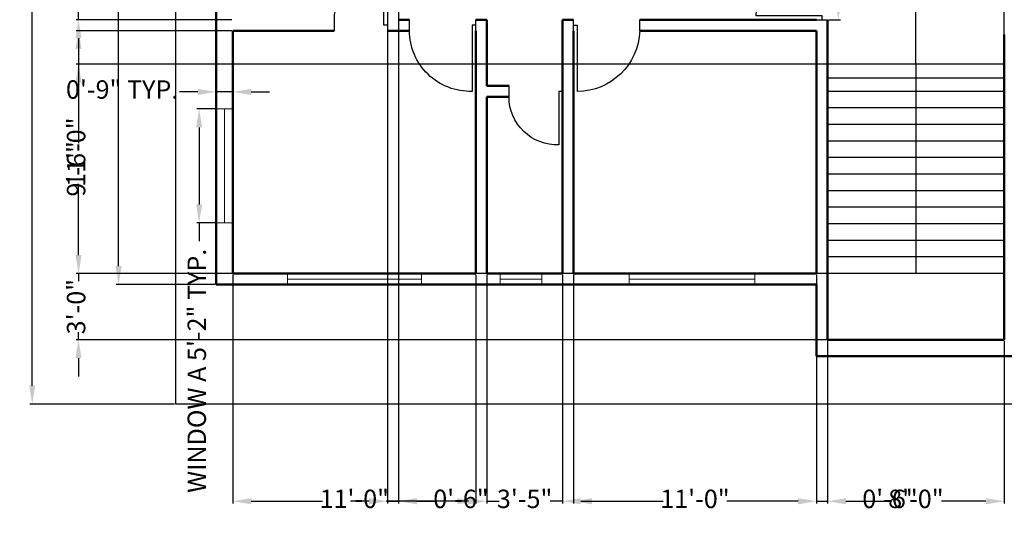
# Model space of a CAD drawing. Units: inches. Extents: x 3237 to 4201, y 2949 to 4053.
# Tile 1 of 5: x 3237 to 3772, y 2949 to 3217. Entities that reach past the tile are written whole.
import ezdxf

# ---------------------------------------------------------------- set-up
doc = ezdxf.new("R2010")
doc.units = ezdxf.units.IN
for name, color, linetype, lineweight in [('A-ANNO-DIMS', 2, 'Continuous', 18), ('A-DOOR', 3, 'Continuous', 25), ('A-FLOR-STRS', 7, 'Continuous', 25), ('A-GLAZ', 4, 'Continuous', 18), ('A-WALL', 7, 'Continuous', 50), ('C-PROP', 6, 'Continuous', 25)]:
    doc.layers.add(name, color=color, linetype=linetype, lineweight=lineweight)
doc.styles.get("Standard").update_dxf_attribs({"font": 'arial.ttf'})
doc.dimstyles.new('ISO-25', dxfattribs={"dimtxt": 10, "dimasz": 10, "dimexe": 1.25, "dimexo": 0.625, "dimtad": 0, "dimdec": 0, "dimlunit": 3, "dimtxsty": 'Standard', "dimcen": 2.5, "dimadec": 0, "dimazin": 0, "dimtfac": 1, "dimtdec": 0, "dimtmove": 0, "dimatfit": 3, "dimfxl": 1, "dimarcsym": 0})

# ---------------------------------------------------------------- blocks, each defined once
blk = doc.blocks.new('*D2')
at = {"layer": 'A-ANNO-DIMS', "color": 0, "lineweight": -2, "transparency": 16777216}
for p, q in [((3320.9, 3907.98), (3242.34, 3907.98)), ((3243.59, 3897.98), (3243.59, 3467.05)), ((3243.59, 3017.98), (3243.59, 3448.91)), ((3320.9, 3007.98), (3242.34, 3007.98))]:
    blk.add_line(p, q, dxfattribs=at)
at = {"layer": 'A-ANNO-DIMS', "color": 0, "transparency": 16777216}
for points in [[(3241.92, 3897.98), (3245.26, 3897.98), (3243.59, 3907.98)], [(3241.92, 3017.98), (3245.26, 3017.98), (3243.59, 3007.98)]]:
    blk.add_solid(points, dxfattribs=at)
at = {"layer": 'Defpoints', "color": 0, "transparency": 16777216}
for p in [(3321.52, 3907.98), (3243.59, 3007.98), (3321.52, 3007.98)]:
    blk.add_point(p, dxfattribs=at)
at = {"layer": 'A-ANNO-DIMS', "color": 0, "transparency": 16777216, "insert": (3243.59, 3457.98), "char_height": 10, "attachment_point": 5, "rotation": 90}
blk.add_mtext("75'", dxfattribs=at)
blk = doc.blocks.new('*D4')
at = {"layer": 'A-ANNO-DIMS', "color": 0, "lineweight": -2, "transparency": 16777216}
for p, q in [((3342.9, 3885.98), (3289.25, 3885.98)), ((3290.5, 3875.98), (3290.5, 3497.31)), ((3290.5, 3082.98), (3290.5, 3461.65)), ((3342.9, 3072.98), (3289.25, 3072.98))]:
    blk.add_line(p, q, dxfattribs=at)
at = {"layer": 'A-ANNO-DIMS', "color": 0, "transparency": 16777216}
for points in [[(3288.84, 3875.98), (3292.17, 3875.98), (3290.5, 3885.98)], [(3288.84, 3082.98), (3292.17, 3082.98), (3290.5, 3072.98)]]:
    blk.add_solid(points, dxfattribs=at)
at = {"layer": 'Defpoints', "color": 0, "transparency": 16777216}
for p in [(3343.52, 3885.98), (3290.5, 3072.98), (3343.52, 3072.98)]:
    blk.add_point(p, dxfattribs=at)
at = {"layer": 'A-ANNO-DIMS', "color": 0, "transparency": 16777216, "insert": (3290.5, 3479.48), "char_height": 10, "attachment_point": 5, "rotation": 90}
blk.add_mtext('67\'-9"', dxfattribs=at)
blk = doc.blocks.new('DOOR-36-OFFSET-A')
for p, q in [((2, 3), (2, 39)), ((0, 6), (0, 0)), ((36, 6), (36, 0)), ((0, 3), (2, 3))]:
    blk.add_line(p, q)
blk.add_arc((2, 4.98), 34.02, 1.7102, 90)
blk = doc.blocks.new('DOOR-29-OFFSET-B')
for p, q in [((27, 3), (27, 32)), ((0, 6), (0, 0)), ((29, 6), (29, 0)), ((29, 3), (27, 3))]:
    blk.add_line(p, q)
blk.add_arc((26.02, 6), 26.02, 87.8382, 180)
blk = doc.blocks.new('DOOR-36-OFFSET-B')
for p, q in [((34, 3), (34, 39)), ((0, 6), (0, 0)), ((36, 6), (36, 0)), ((36, 3), (34, 3))]:
    blk.add_line(p, q)
blk.add_arc((33.01, 6), 33.01, 88.2898, 180)
blk = doc.blocks.new('WIN-61p86IN')
for p, q in [((0, 61.86), (9, 61.86)), ((4.5, 0), (4.5, 61.86)), ((0, 0), (9, 0))]:
    blk.add_line(p, q)
blk = doc.blocks.new('*D22')
at = {"layer": 'A-ANNO-DIMS', "color": 0, "lineweight": -2, "transparency": 16777216}
for p, q in [((3681.37, 3252.98), (3681.37, 3262.98)), ((3676.15, 3252.98), (3682.62, 3252.98)), ((3681.37, 3226.98), (3681.37, 3242.98)), ((3676.15, 3216.98), (3682.62, 3216.98))]:
    blk.add_line(p, q, dxfattribs=at)
at = {"layer": 'A-ANNO-DIMS', "color": 0, "transparency": 16777216}
for points in [[(3679.71, 3242.98), (3683.04, 3242.98), (3681.37, 3252.98)], [(3679.71, 3226.98), (3683.04, 3226.98), (3681.37, 3216.98)]]:
    blk.add_solid(points, dxfattribs=at)
at = {"layer": 'Defpoints', "color": 0, "transparency": 16777216}
for p in [(3675.52, 3252.98), (3681.37, 3252.98), (3675.52, 3216.98)]:
    blk.add_point(p, dxfattribs=at)
at = {"layer": 'A-ANNO-DIMS', "color": 0, "transparency": 16777216, "insert": (3681.37, 3294.08), "char_height": 10, "attachment_point": 5, "rotation": 90}
blk.add_mtext('3\'-0" TYP.', dxfattribs=at)
blk = doc.blocks.new('*D27')
at = {"layer": 'A-ANNO-DIMS', "color": 0, "lineweight": -2, "transparency": 16777216}
for p, q in [((3342.9, 3168.43), (3332.99, 3168.43)), ((3334.24, 3158.43), (3334.24, 3116.57)), ((3342.9, 3106.57), (3332.99, 3106.57)), ((3334.24, 3106.57), (3334.24, 3096.57))]:
    blk.add_line(p, q, dxfattribs=at)
at = {"layer": 'A-ANNO-DIMS', "color": 0, "transparency": 16777216}
for points in [[(3332.58, 3158.43), (3335.91, 3158.43), (3334.24, 3168.43)], [(3332.58, 3116.57), (3335.91, 3116.57), (3334.24, 3106.57)]]:
    blk.add_solid(points, dxfattribs=at)
at = {"layer": 'Defpoints', "color": 0, "transparency": 16777216}
for p in [(3343.52, 3168.43), (3334.24, 3106.57), (3343.52, 3106.57)]:
    blk.add_point(p, dxfattribs=at)
at = {"layer": 'A-ANNO-DIMS', "color": 0, "transparency": 16777216, "insert": (3334.24, 3026.08), "char_height": 10, "attachment_point": 5, "rotation": 90}
blk.add_mtext('WINDOW A 5\'-2" TYP.', dxfattribs=at)
blk = doc.blocks.new('*D28')
at = {"layer": 'A-ANNO-DIMS', "color": 0, "lineweight": -2, "transparency": 16777216}
for p, q in [((3333.52, 3177.71), (3323.52, 3177.71)), ((3343.52, 3169.05), (3343.52, 3178.96)), ((3352.52, 3177.71), (3343.52, 3177.71)), ((3352.52, 3169.05), (3352.52, 3178.96)), ((3362.52, 3177.71), (3372.52, 3177.71))]:
    blk.add_line(p, q, dxfattribs=at)
at = {"layer": 'A-ANNO-DIMS', "color": 0, "transparency": 16777216}
for points in [[(3333.52, 3179.37), (3333.52, 3176.04), (3343.52, 3177.71)], [(3362.52, 3179.37), (3362.52, 3176.04), (3352.52, 3177.71)]]:
    blk.add_solid(points, dxfattribs=at)
at = {"layer": 'Defpoints', "color": 0, "transparency": 16777216}
for p in [(3343.52, 3177.71), (3343.52, 3168.43), (3352.52, 3168.43)]:
    blk.add_point(p, dxfattribs=at)
at = {"layer": 'A-ANNO-DIMS', "color": 0, "transparency": 16777216, "insert": (3292.42, 3177.71), "char_height": 10, "attachment_point": 5}
blk.add_mtext('0\'-9" TYP.', dxfattribs=at)
blk = doc.blocks.new('*D53')
at = {"layer": 'A-ANNO-DIMS', "color": 0, "lineweight": -2, "transparency": 16777216}
for p, q in [((3352.52, 3078.35), (3352.52, 2953.93)), ((3484.52, 3078.35), (3484.52, 2953.93)), ((3362.52, 2955.18), (3401.19, 2955.18)), ((3474.52, 2955.18), (3435.85, 2955.18))]:
    blk.add_line(p, q, dxfattribs=at)
at = {"layer": 'A-ANNO-DIMS', "color": 0, "transparency": 16777216}
for points in [[(3362.52, 2956.85), (3362.52, 2953.51), (3352.52, 2955.18)], [(3474.52, 2956.85), (3474.52, 2953.51), (3484.52, 2955.18)]]:
    blk.add_solid(points, dxfattribs=at)
at = {"layer": 'Defpoints', "color": 0, "transparency": 16777216}
for p in [(3352.52, 3078.98), (3484.52, 3078.98), (3484.52, 2955.18)]:
    blk.add_point(p, dxfattribs=at)
at = {"layer": 'A-ANNO-DIMS', "color": 0, "transparency": 16777216, "insert": (3418.52, 2955.18), "char_height": 10, "attachment_point": 5}
blk.add_mtext('11\'-0"', dxfattribs=at)
blk = doc.blocks.new('*D54')
at = {"layer": 'A-ANNO-DIMS', "color": 0, "lineweight": -2, "transparency": 16777216}
for p, q in [((3490.52, 3078.35), (3490.52, 2953.93)), ((3531.52, 3078.35), (3531.52, 2953.93)), ((3480.52, 2955.18), (3470.52, 2955.18)), ((3490.52, 2955.18), (3497.11, 2955.18)), ((3531.52, 2955.18), (3524.93, 2955.18)), ((3541.52, 2955.18), (3551.52, 2955.18))]:
    blk.add_line(p, q, dxfattribs=at)
at = {"layer": 'A-ANNO-DIMS', "color": 0, "transparency": 16777216}
for points in [[(3480.52, 2956.85), (3480.52, 2953.51), (3490.52, 2955.18)], [(3541.52, 2956.85), (3541.52, 2953.51), (3531.52, 2955.18)]]:
    blk.add_solid(points, dxfattribs=at)
at = {"layer": 'Defpoints', "color": 0, "transparency": 16777216}
for p in [(3490.52, 3078.98), (3531.52, 3078.98), (3531.52, 2955.18)]:
    blk.add_point(p, dxfattribs=at)
at = {"layer": 'A-ANNO-DIMS', "color": 0, "transparency": 16777216, "insert": (3511.02, 2955.18), "char_height": 10, "attachment_point": 5}
blk.add_mtext('3\'-5"', dxfattribs=at)
blk = doc.blocks.new('*D55')
at = {"layer": 'A-ANNO-DIMS', "color": 0, "lineweight": -2, "transparency": 16777216}
for p, q in [((3537.52, 3078.35), (3537.52, 2953.93)), ((3669.52, 3078.35), (3669.52, 2953.93)), ((3547.52, 2955.18), (3586.19, 2955.18)), ((3659.52, 2955.18), (3620.85, 2955.18))]:
    blk.add_line(p, q, dxfattribs=at)
at = {"layer": 'A-ANNO-DIMS', "color": 0, "transparency": 16777216}
for points in [[(3547.52, 2956.85), (3547.52, 2953.51), (3537.52, 2955.18)], [(3659.52, 2956.85), (3659.52, 2953.51), (3669.52, 2955.18)]]:
    blk.add_solid(points, dxfattribs=at)
at = {"layer": 'Defpoints', "color": 0, "transparency": 16777216}
for p in [(3537.52, 3078.98), (3669.52, 3078.98), (3669.52, 2955.18)]:
    blk.add_point(p, dxfattribs=at)
at = {"layer": 'A-ANNO-DIMS', "color": 0, "transparency": 16777216, "insert": (3603.52, 2955.18), "char_height": 10, "attachment_point": 5}
blk.add_mtext('11\'-0"', dxfattribs=at)
blk = doc.blocks.new('*D59')
at = {"layer": 'A-ANNO-DIMS', "color": 0, "lineweight": -2, "transparency": 16777216}
for p, q in [((3351.9, 3210.98), (3267.47, 3210.98)), ((3268.72, 3200.98), (3268.72, 3162.31)), ((3268.72, 3088.98), (3268.72, 3127.65)), ((3351.9, 3078.98), (3267.47, 3078.98))]:
    blk.add_line(p, q, dxfattribs=at)
at = {"layer": 'A-ANNO-DIMS', "color": 0, "transparency": 16777216}
for points in [[(3267.06, 3200.98), (3270.39, 3200.98), (3268.72, 3210.98)], [(3267.06, 3088.98), (3270.39, 3088.98), (3268.72, 3078.98)]]:
    blk.add_solid(points, dxfattribs=at)
at = {"layer": 'Defpoints', "color": 0, "transparency": 16777216}
for p in [(3268.72, 3210.98), (3352.52, 3210.98), (3352.52, 3078.98)]:
    blk.add_point(p, dxfattribs=at)
at = {"layer": 'A-ANNO-DIMS', "color": 0, "transparency": 16777216, "insert": (3268.72, 3144.98), "char_height": 10, "attachment_point": 5, "rotation": 90}
blk.add_mtext('11\'-0"', dxfattribs=at)
blk = doc.blocks.new('*D60')
at = {"layer": 'A-ANNO-DIMS', "color": 0, "lineweight": -2, "transparency": 16777216}
for p, q in [((3268.72, 3270.98), (3268.72, 3280.98)), ((3351.9, 3260.98), (3267.47, 3260.98)), ((3268.72, 3260.98), (3268.72, 3252.89)), ((3268.72, 3216.98), (3268.72, 3225.07)), ((3351.9, 3216.98), (3267.47, 3216.98)), ((3268.72, 3206.98), (3268.72, 3196.98))]:
    blk.add_line(p, q, dxfattribs=at)
at = {"layer": 'A-ANNO-DIMS', "color": 0, "transparency": 16777216}
for points in [[(3267.06, 3270.98), (3270.39, 3270.98), (3268.72, 3260.98)], [(3267.06, 3206.98), (3270.39, 3206.98), (3268.72, 3216.98)]]:
    blk.add_solid(points, dxfattribs=at)
at = {"layer": 'Defpoints', "color": 0, "transparency": 16777216}
for p in [(3268.72, 3260.98), (3352.52, 3260.98), (3352.52, 3216.98)]:
    blk.add_point(p, dxfattribs=at)
at = {"layer": 'A-ANNO-DIMS', "color": 0, "transparency": 16777216, "insert": (3268.72, 3238.98), "char_height": 10, "attachment_point": 5, "rotation": 90}
blk.add_mtext('3\'-8"', dxfattribs=at)
blk = doc.blocks.new('*D75')
at = {"layer": 'A-ANNO-DIMS', "color": 0, "lineweight": -2, "transparency": 16777216}
for p, q in [((3436.52, 3266.35), (3436.52, 2953.93)), ((3442.52, 3266.35), (3442.52, 2953.93)), ((3426.52, 2955.18), (3416.52, 2955.18)), ((3436.52, 2955.18), (3442.52, 2955.18)), ((3452.52, 2955.18), (3462.52, 2955.18))]:
    blk.add_line(p, q, dxfattribs=at)
at = {"layer": 'A-ANNO-DIMS', "color": 0, "transparency": 16777216}
for points in [[(3426.52, 2956.85), (3426.52, 2953.51), (3436.52, 2955.18)], [(3452.52, 2956.85), (3452.52, 2953.51), (3442.52, 2955.18)]]:
    blk.add_solid(points, dxfattribs=at)
at = {"layer": 'Defpoints', "color": 0, "transparency": 16777216}
for p in [(3436.52, 3266.98), (3442.52, 3266.98), (3442.52, 2955.18)]:
    blk.add_point(p, dxfattribs=at)
at = {"layer": 'A-ANNO-DIMS', "color": 0, "transparency": 16777216, "insert": (3476.44, 2955.18), "char_height": 10, "attachment_point": 5}
blk.add_mtext('0\'-6"', dxfattribs=at)
blk = doc.blocks.new('*D80')
at = {"layer": 'A-ANNO-DIMS', "color": 0, "lineweight": -2, "transparency": 16777216}
for p, q in [((3675.52, 3042.35), (3675.52, 2953.93)), ((3771.52, 3042.35), (3771.52, 2953.93)), ((3685.52, 2955.18), (3709.6, 2955.18)), ((3761.52, 2955.18), (3737.44, 2955.18))]:
    blk.add_line(p, q, dxfattribs=at)
at = {"layer": 'A-ANNO-DIMS', "color": 0, "transparency": 16777216}
for points in [[(3685.52, 2956.85), (3685.52, 2953.51), (3675.52, 2955.18)], [(3761.52, 2956.85), (3761.52, 2953.51), (3771.52, 2955.18)]]:
    blk.add_solid(points, dxfattribs=at)
at = {"layer": 'Defpoints', "color": 0, "transparency": 16777216}
for p in [(3675.52, 3042.98), (3771.52, 3042.98), (3771.52, 2955.18)]:
    blk.add_point(p, dxfattribs=at)
at = {"layer": 'A-ANNO-DIMS', "color": 0, "transparency": 16777216, "insert": (3723.52, 2955.18), "char_height": 10, "attachment_point": 5}
blk.add_mtext('8\'-0"', dxfattribs=at)
blk = doc.blocks.new('*D81')
at = {"layer": 'A-ANNO-DIMS', "color": 0, "lineweight": -2, "transparency": 16777216}
for p, q in [((3268.72, 3088.98), (3268.72, 3098.98)), ((3674.9, 3078.98), (3267.47, 3078.98)), ((3268.72, 3078.98), (3268.72, 3074.89)), ((3674.9, 3042.98), (3267.47, 3042.98)), ((3268.72, 3042.98), (3268.72, 3047.07)), ((3268.72, 3032.98), (3268.72, 3022.98))]:
    blk.add_line(p, q, dxfattribs=at)
at = {"layer": 'A-ANNO-DIMS', "color": 0, "transparency": 16777216}
for points in [[(3267.06, 3088.98), (3270.39, 3088.98), (3268.72, 3078.98)], [(3267.06, 3032.98), (3270.39, 3032.98), (3268.72, 3042.98)]]:
    blk.add_solid(points, dxfattribs=at)
at = {"layer": 'Defpoints', "color": 0, "transparency": 16777216}
for p in [(3675.52, 3078.98), (3268.72, 3042.98), (3675.52, 3042.98)]:
    blk.add_point(p, dxfattribs=at)
at = {"layer": 'A-ANNO-DIMS', "color": 0, "transparency": 16777216, "insert": (3268.72, 3060.98), "char_height": 10, "attachment_point": 5, "rotation": 90}
blk.add_mtext('3\'-0"', dxfattribs=at)
blk = doc.blocks.new('*D82')
at = {"layer": 'A-ANNO-DIMS', "color": 0, "lineweight": -2, "transparency": 16777216}
for p, q in [((3674.9, 3192.78), (3267.47, 3192.78)), ((3268.72, 3182.78), (3268.72, 3149.79)), ((3268.72, 3088.98), (3268.72, 3121.96)), ((3674.9, 3078.98), (3267.47, 3078.98))]:
    blk.add_line(p, q, dxfattribs=at)
at = {"layer": 'A-ANNO-DIMS', "color": 0, "transparency": 16777216}
for points in [[(3267.06, 3182.78), (3270.39, 3182.78), (3268.72, 3192.78)], [(3267.06, 3088.98), (3270.39, 3088.98), (3268.72, 3078.98)]]:
    blk.add_solid(points, dxfattribs=at)
at = {"layer": 'Defpoints', "color": 0, "transparency": 16777216}
for p in [(3268.72, 3192.78), (3675.52, 3192.78), (3675.52, 3078.98)]:
    blk.add_point(p, dxfattribs=at)
at = {"layer": 'A-ANNO-DIMS', "color": 0, "transparency": 16777216, "insert": (3268.72, 3135.88), "char_height": 10, "attachment_point": 5, "rotation": 90}
blk.add_mtext('9\'-6"', dxfattribs=at)
blk = doc.blocks.new('*D83')
at = {"layer": 'A-ANNO-DIMS', "color": 0, "lineweight": -2, "transparency": 16777216}
for p, q in [((3713.52, 3960.78), (3703.52, 3960.78)), ((3723.52, 3193.4), (3723.52, 3962.03)), ((3723.52, 3960.78), (3733.4, 3960.78)), ((3771.52, 3960.78), (3761.64, 3960.78)), ((3771.52, 3193.4), (3771.52, 3962.03)), ((3781.52, 3960.78), (3791.52, 3960.78))]:
    blk.add_line(p, q, dxfattribs=at)
at = {"layer": 'A-ANNO-DIMS', "color": 0, "transparency": 16777216}
for points in [[(3713.52, 3962.45), (3713.52, 3959.11), (3723.52, 3960.78)], [(3781.52, 3962.45), (3781.52, 3959.11), (3771.52, 3960.78)]]:
    blk.add_solid(points, dxfattribs=at)
at = {"layer": 'Defpoints', "color": 0, "transparency": 16777216}
for p in [(3771.52, 3960.78), (3723.52, 3192.78), (3771.52, 3192.78)]:
    blk.add_point(p, dxfattribs=at)
at = {"layer": 'A-ANNO-DIMS', "color": 0, "transparency": 16777216, "insert": (3747.52, 3960.78), "char_height": 10, "attachment_point": 5}
blk.add_mtext('4\'-0"', dxfattribs=at)
blk = doc.blocks.new('*D86')
at = {"layer": 'A-ANNO-DIMS', "color": 0, "lineweight": -2, "transparency": 16777216}
for p, q in [((3675.52, 3042.35), (3675.52, 2953.93)), ((3669.52, 3033.35), (3669.52, 2953.93)), ((3659.52, 2955.18), (3649.52, 2955.18)), ((3669.52, 2955.18), (3675.52, 2955.18)), ((3685.52, 2955.18), (3695.52, 2955.18))]:
    blk.add_line(p, q, dxfattribs=at)
at = {"layer": 'A-ANNO-DIMS', "color": 0, "transparency": 16777216}
for points in [[(3659.52, 2956.85), (3659.52, 2953.51), (3669.52, 2955.18)], [(3685.52, 2956.85), (3685.52, 2953.51), (3675.52, 2955.18)]]:
    blk.add_solid(points, dxfattribs=at)
at = {"layer": 'Defpoints', "color": 0, "transparency": 16777216}
for p in [(3675.52, 3042.98), (3669.52, 3033.98), (3675.52, 2955.18)]:
    blk.add_point(p, dxfattribs=at)
at = {"layer": 'A-ANNO-DIMS', "color": 0, "transparency": 16777216, "insert": (3709.44, 2955.18), "char_height": 10, "attachment_point": 5}
blk.add_mtext('0\'-6"', dxfattribs=at)

msp = doc.modelspace()

# ---------------------------------------------------------------- linework, layer by layer
at = {"layer": 'A-FLOR-STRS'}
for p, q in [((3771.52, 3192.78), (3675.52, 3192.78)), ((3723.52, 3192.78), (3723.52, 3078.98)), ((3771.52, 3185.23), (3675.52, 3185.23)), ((3771.52, 3177.98), (3675.52, 3177.98)), ((3771.52, 3168.98), (3675.52, 3168.98)), ((3771.52, 3159.98), (3675.52, 3159.98)), ((3771.52, 3150.98), (3675.52, 3150.98)), ((3771.52, 3141.98), (3675.52, 3141.98)), ((3771.52, 3132.98), (3675.52, 3132.98)), ((3771.52, 3123.98), (3675.52, 3123.98)), ((3771.52, 3114.98), (3675.52, 3114.98)), ((3771.52, 3105.98), (3675.52, 3105.98)), ((3771.52, 3096.98), (3675.52, 3096.98)), ((3771.52, 3087.98), (3675.52, 3087.98)), ((3771.52, 3078.98), (3675.52, 3078.98))]:
    msp.add_line(p, q, dxfattribs=at)
at = {"layer": 'A-GLAZ'}
for p, q in [((3343.52, 3106.57), (3343.52, 3168.43)), ((3352.52, 3168.43), (3348.02, 3168.43)), ((3382.15, 3078.98), (3382.15, 3072.98)), ((3382.15, 3075.98), (3455, 3075.98)), ((3455, 3078.98), (3455, 3072.98)), ((3497.76, 3078.98), (3497.76, 3072.98)), ((3497.76, 3075.98), (3520.28, 3075.98)), ((3520.28, 3078.98), (3520.28, 3072.98)), ((3567.81, 3078.98), (3567.81, 3072.98)), ((3567.81, 3075.98), (3636.09, 3075.98)), ((3636.09, 3078.98), (3636.09, 3072.98))]:
    msp.add_line(p, q, dxfattribs=at)
at = {"layer": 'A-WALL'}
for p, q in [((3343.52, 3598.98), (3343.52, 3072.98)), ((3448.52, 3216.98), (3442.52, 3216.98)), ((3484.52, 3216.98), (3490.52, 3216.98)), ((3490.52, 3216.98), (3490.52, 3208.98)), ((3531.52, 3208.98), (3531.52, 3216.98)), ((3531.52, 3216.98), (3537.52, 3216.98)), ((3537.52, 3216.98), (3531.52, 3216.98)), ((3669.52, 3216.98), (3573.52, 3216.98)), ((3675.52, 3216.98), (3675.52, 3078.98)), ((3352.52, 3210.98), (3352.52, 3078.98)), ((3407.52, 3210.98), (3352.52, 3210.98)), ((3448.52, 3210.98), (3436.52, 3210.98)), ((3484.52, 3210.98), (3484.52, 3078.98)), ((3484.52, 3210.98), (3484.52, 3078.98)), ((3490.52, 3202.98), (3490.52, 3208.98)), ((3531.52, 3208.98), (3531.52, 3078.98)), ((3537.52, 3210.98), (3537.52, 3208.98)), ((3537.52, 3208.98), (3537.52, 3078.98)), ((3669.52, 3210.98), (3573.52, 3210.98)), ((3669.52, 3210.98), (3669.52, 3208.98)), ((3669.52, 3208.98), (3669.52, 3201.96)), ((3771.52, 3208.98), (3771.52, 3078.98)), ((3490.52, 3202.98), (3490.52, 3180.98)), ((3669.52, 3202.98), (3669.52, 3078.98)), ((3502.52, 3180.98), (3490.52, 3180.98)), ((3502.52, 3174.98), (3490.52, 3174.98)), ((3490.52, 3174.98), (3490.52, 3078.98)), ((3771.52, 3042.98), (3771.52, 3085.51)), ((3484.52, 3078.98), (3352.52, 3078.98)), ((3531.52, 3078.98), (3490.52, 3078.98)), ((3669.52, 3078.98), (3537.52, 3078.98)), ((3675.52, 3078.98), (3675.52, 3042.98)), ((3352.52, 3072.98), (3343.52, 3072.98)), ((3669.52, 3072.98), (3352.52, 3072.98)), ((3669.52, 3072.98), (3669.52, 3042.98)), ((3669.52, 3042.98), (3669.52, 3033.98)), ((3675.52, 3042.98), (3771.52, 3042.98)), ((3669.52, 3033.98), (3771.38, 3033.98)), ((3771.38, 3033.98), (3777.38, 3033.98))]:
    msp.add_line(p, q, dxfattribs=at)
at = {"layer": 'C-PROP'}
for p, q in [((3321.52, 3007.98), (3321.52, 3907.98)), ((3343.52, 3007.98), (3321.52, 3007.98)), ((3353.52, 3007.98), (3343.52, 3007.98)), ((4133.52, 3007.98), (3353.52, 3007.98))]:
    msp.add_line(p, q, dxfattribs=at)

# ---------------------------------------------------------------- block references
at = {"layer": 'A-DOOR', "rotation": 89.99999999999756}
msp.add_blockref('DOOR-36-OFFSET-A', (3675.52, 3216.98), dxfattribs=at)
at = {"layer": 'A-DOOR'}
msp.add_blockref('DOOR-29-OFFSET-B', (3407.52, 3210.98), dxfattribs=at)
at = {"layer": 'A-DOOR', "extrusion": (0, 0, -1), "zscale": -1, "rotation": 180}
for name, p in [('DOOR-36-OFFSET-B', (-3448.52, 3216.98)), ('DOOR-36-OFFSET-A', (-3537.52, 3216.98)), ('DOOR-29-OFFSET-B', (-3502.52, 3180.98))]:
    msp.add_blockref(name, p, dxfattribs=at)
at = {"layer": 'A-GLAZ', "rotation": 180}
msp.add_blockref('WIN-61p86IN', (3352.52, 3168.43), dxfattribs=at)

# ---------------------------------------------------------------- dimensions: what is measured, and where the dimension line sits
at = {"layer": 'A-ANNO-DIMS'}
for base, p1, p2, picture, middle in [((3771.52, 3960.78), (3723.52, 3192.78), (3771.52, 3192.78), '*D83', (3747.52, 3960.78)), ((3442.52, 2955.18), (3436.52, 3266.98), (3442.52, 3266.98), '*D75', (3476.44, 2955.18)), ((3484.52, 2955.18), (3352.52, 3078.98), (3484.52, 3078.98), '*D53', (3418.52, 2955.18)), ((3531.52, 2955.18), (3490.52, 3078.98), (3531.52, 3078.98), '*D54', (3511.02, 2955.18)), ((3669.52, 2955.18), (3537.52, 3078.98), (3669.52, 3078.98), '*D55', (3603.52, 2955.18)), ((3675.52, 2955.18), (3669.52, 3033.98), (3675.52, 3042.98), '*D86', (3709.44, 2955.18)), ((3771.52, 2955.18), (3675.52, 3042.98), (3771.52, 3042.98), '*D80', (3723.52, 2955.18))]:
    dim = msp.add_linear_dim(base=base, p1=p1, p2=p2, dimstyle='ISO-25', override={"dimdec": 1, "dimlfac": 1, "dimrnd": 0, "dimzin": 1, "dimdsep": 46, "dimlunit": 4, "dimfrac": 2}, dxfattribs=at)
    dim.commit()
    dim.dimension.update_dxf_attribs({"geometry": picture, "text_midpoint": middle})
for base, p1, p2, override, picture, middle in [((3243.59, 3007.98), (3321.52, 3907.98), (3321.52, 3007.98), {"dimclrd": 0, "dimclre": 0, "dimclrt": 0}, '*D2', (3243.59, 3457.98)), ((3290.5, 3072.98), (3343.52, 3885.98), (3343.52, 3072.98), {"dimclrd": 0, "dimclre": 0, "dimclrt": 0}, '*D4', (3290.5, 3479.48)), ((3268.72, 3260.98), (3352.52, 3216.98), (3352.52, 3260.98), {"dimdec": 1, "dimlfac": 1, "dimrnd": 0, "dimzin": 1, "dimdsep": 46, "dimlunit": 4, "dimfrac": 2}, '*D60', (3268.72, 3238.98)), ((3268.72, 3210.98), (3352.52, 3078.98), (3352.52, 3210.98), {"dimdec": 1, "dimlfac": 1, "dimrnd": 0, "dimzin": 1, "dimdsep": 46, "dimlunit": 4, "dimfrac": 2}, '*D59', (3268.72, 3144.98)), ((3268.72, 3192.78), (3675.52, 3078.98), (3675.52, 3192.78), {"dimdec": 1, "dimlfac": 1, "dimrnd": 0, "dimzin": 1, "dimdsep": 46, "dimlunit": 4, "dimfrac": 2}, '*D82', (3268.72, 3135.88)), ((3268.72, 3042.98), (3675.52, 3078.98), (3675.52, 3042.98), {"dimdec": 1, "dimlfac": 1, "dimrnd": 0, "dimzin": 1, "dimdsep": 46, "dimlunit": 4, "dimfrac": 2}, '*D81', (3268.72, 3060.98))]:
    dim = msp.add_linear_dim(base=base, p1=p1, p2=p2, angle=90, dimstyle='ISO-25', override=override, dxfattribs=at)
    dim.commit()
    dim.dimension.update_dxf_attribs({"geometry": picture, "text_midpoint": middle})
for base, p1, p2, angle, text, picture, middle in [((3681.37, 3252.98), (3675.52, 3216.98), (3675.52, 3252.98), 90, '<> TYP.', '*D22', (3681.37, 3294.08)), ((3343.52, 3177.71), (3352.52, 3168.43), (3343.52, 3168.43), 180, '<> TYP.', '*D28', (3292.42, 3177.71)), ((3334.24, 3106.57), (3343.52, 3168.43), (3343.52, 3106.57), 270, 'WINDOW A <> TYP.', '*D27', (3334.24, 3026.08))]:
    dim = msp.add_linear_dim(base=base, p1=p1, p2=p2, angle=angle, text=text, dimstyle='ISO-25', override={"dimdec": 1, "dimlfac": 1, "dimrnd": 0, "dimzin": 1, "dimdsep": 46, "dimlunit": 4, "dimfrac": 2}, dxfattribs=at)
    dim.commit()
    dim.dimension.update_dxf_attribs({"geometry": picture, "text_midpoint": middle})

doc.saveas('drawing.dxf')
